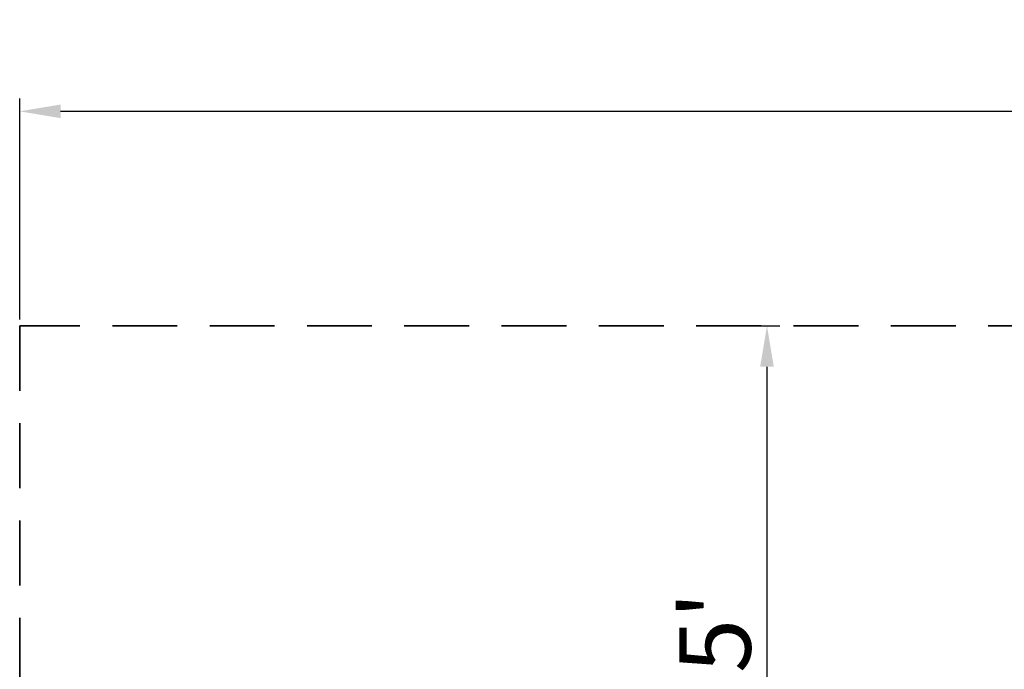
# Model space of a CAD drawing. Units: inches. Extents: x -7 to 1228, y -146 to 1091.
# Tile 54 of 88: x 0 to 96, y 1027 to 1091. Entities that reach past the tile are written whole.
import ezdxf

# ---------------------------------------------------------------- set-up
doc = ezdxf.new("R2010")
doc.units = ezdxf.units.IN
doc.linetypes.add('DASHED2', pattern=[9.525, 6.35, -3.175])
doc.layers.add('A-ANNO-DIMS', color=2, linetype='Continuous', lineweight=18)
doc.layers.add('C-PROP', color=1, linetype='DASHED2', lineweight=35)
doc.styles.get("Standard").update_dxf_attribs({"font": 'arial.ttf'})
doc.dimstyles.new('ISO-25', dxfattribs={"dimtxt": 7, "dimasz": 4, "dimexe": 1.25, "dimexo": 0.625, "dimtad": 1, "dimdec": 1, "dimlunit": 3, "dimtxsty": 'Standard', "dimcen": 2.5, "dimadec": 0, "dimazin": 0, "dimtfac": 1, "dimtdec": 1, "dimtmove": 1, "dimatfit": 3, "dimfxl": 1, "dimarcsym": 0})

# ---------------------------------------------------------------- blocks, each defined once
blk = doc.blocks.new('*D11')
at = {"layer": 'A-ANNO-DIMS', "color": 0, "lineweight": -2, "transparency": 16777216}
for p, q in [((0, 1061.625), (0, 1083.25)), ((1187, 1061.625), (1187, 1083.25)), ((4, 1082), (1183, 1082))]:
    blk.add_line(p, q, dxfattribs=at)
at = {"layer": 'A-ANNO-DIMS', "color": 0, "transparency": 16777216}
for points in [[(4, 1082.667), (4, 1081.333), (0, 1082)], [(1183, 1082.667), (1183, 1081.333), (1187, 1082)]]:
    blk.add_solid(points, dxfattribs=at)
at = {"layer": 'Defpoints', "color": 0, "transparency": 16777216}
for p in [(1187, 1082), (0, 1061), (1187, 1061)]:
    blk.add_point(p, dxfattribs=at)
at = {"layer": 'A-ANNO-DIMS', "color": 0, "transparency": 16777216, "insert": (593.5, 1086.199), "char_height": 7, "attachment_point": 5}
blk.add_mtext('98\'-11"', dxfattribs=at)
blk = doc.blocks.new('*D15')
at = {"layer": 'A-ANNO-DIMS', "color": 0, "lineweight": -2, "transparency": 16777216}
for p, q in [((68.951, 1061), (74.399, 1061)), ((73.149, 1057), (73.149, 1005)), ((68.951, 1001), (74.399, 1001))]:
    blk.add_line(p, q, dxfattribs=at)
at = {"layer": 'A-ANNO-DIMS', "color": 0, "transparency": 16777216}
for points in [[(72.482, 1057), (73.815, 1057), (73.149, 1061)], [(72.482, 1005), (73.815, 1005), (73.149, 1001)]]:
    blk.add_solid(points, dxfattribs=at)
at = {"layer": 'Defpoints', "color": 0, "transparency": 16777216}
for p in [(68.326, 1061), (68.326, 1001), (73.149, 1001)]:
    blk.add_point(p, dxfattribs=at)
at = {"layer": 'A-ANNO-DIMS', "color": 0, "transparency": 16777216, "insert": (68.964, 1031), "char_height": 7, "attachment_point": 5, "rotation": 90}
blk.add_mtext("5'", dxfattribs=at)

msp = doc.modelspace()

# ---------------------------------------------------------------- linework, layer by layer
at = {"layer": 'C-PROP'}
for p, q in [((1187, 1061), (0, 1061)), ((0, 1061), (0, 0))]:
    msp.add_line(p, q, dxfattribs=at)

# ---------------------------------------------------------------- dimensions: what is measured, and where the dimension line sits
at = {"layer": 'A-ANNO-DIMS'}
dim = msp.add_linear_dim(base=(1187, 1082), p1=(0, 1061), p2=(1187, 1061), dimstyle='ISO-25', override={"dimclrd": 0, "dimclre": 0, "dimclrt": 0}, dxfattribs=at)
dim.commit()
dim.dimension.update_dxf_attribs({"geometry": '*D11', "text_midpoint": (593.5, 1086.199)})
dim = msp.add_linear_dim(base=(73.149, 1001), p1=(68.326, 1061), p2=(68.326, 1001), angle=90, dimstyle='ISO-25', override={"dimclrd": 0, "dimclre": 0, "dimclrt": 0}, dxfattribs=at)
dim.commit()
dim.dimension.update_dxf_attribs({"geometry": '*D15', "text_midpoint": (68.964, 1031)})

doc.saveas('drawing.dxf')
